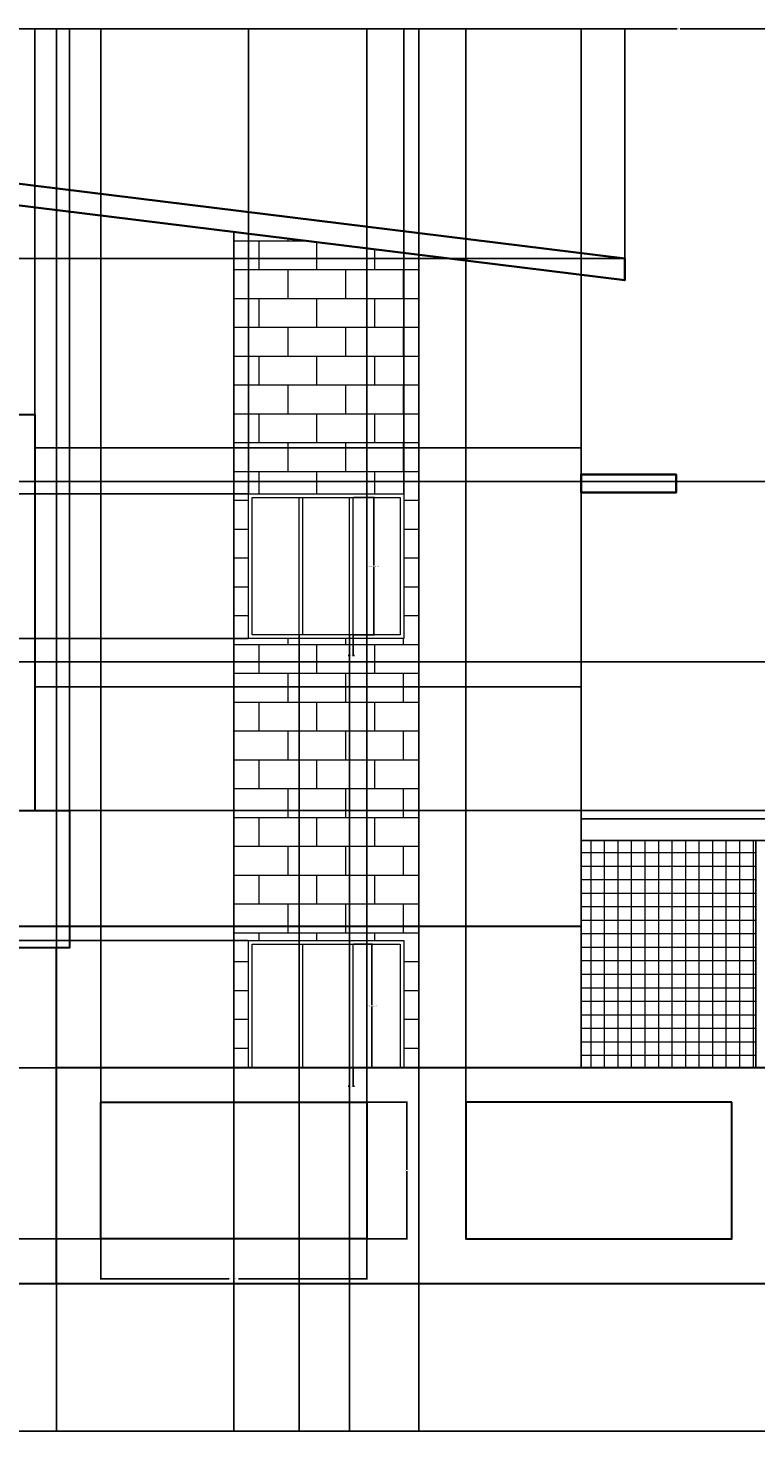
# Model space of a CAD drawing. Units: inches. Extents: x -14 to 886, y 45 to 435.
# Tile 4 of 5: x 384 to 586, y 45 to 435. Entities that reach past the tile are written whole.
import ezdxf

# ---------------------------------------------------------------- set-up
doc = ezdxf.new("R2010")
doc.units = ezdxf.units.IN
doc.header["$MEASUREMENT"] = 0
for name, color, linetype, lineweight in [('A-ANNO-DIMS', 2, 'Continuous', 18), ('A-ELEV-BAND', 7, 'Continuous', 30), ('A-ELEV-PATT', 252, 'Continuous', 13), ('A-GLAZ', 4, 'Continuous', 18), ('A-ROOF', 7, 'Continuous', 35), ('A-WALL', 7, 'Continuous', 25), ('A-WALL-PATT', 252, 'Continuous', 13), ('L-WALL', 7, 'Continuous', 30)]:
    doc.layers.add(name, color=color, linetype=linetype, lineweight=lineweight)
doc.styles.get("Standard").update_dxf_attribs({"font": 'arial.ttf'})
doc.dimstyles.get("Standard").update_dxf_attribs({"dimtxt": 0.18, "dimasz": 0.18, "dimexe": 0.18, "dimexo": 0.0625, "dimgap": 0.09, "dimtad": 0, "dimtih": 1, "dimtoh": 1, "dimdec": 4, "dimzin": 0, "dimdsep": 46, "dimtxsty": 'Standard', "dimcen": 0.09, "dimadec": 0, "dimazin": 0, "dimtfac": 1, "dimtdec": 4, "dimtofl": 0, "dimtmove": 0, "dimatfit": 3, "dimfxl": 1, "dimtolj": 1, "dimtzin": 0, "dimarcsym": 0})

# ---------------------------------------------------------------- blocks, each defined once
blk = doc.blocks.new('BOUNDARY-WALL-INSET')
blk.add_lwpolyline([(0, 37.91), (73.78, 37.91), (73.78, 0), (0, 0)], close=True)
blk = doc.blocks.new('MULLION-UPPER')
for p, q in [((0, 0), (0, 38.1)), ((1, 0), (1, 38.1))]:
    blk.add_line(p, q)
blk = doc.blocks.new('MULLION-LOWER')
for p, q in [((0, 0), (0, 34.29)), ((1, 0), (1, 34.29))]:
    blk.add_line(p, q)
blk = doc.blocks.new('*D10')
at = {"layer": 'A-ANNO-DIMS', "color": 0, "lineweight": -2, "transparency": 16777216}
for p, q in [((404.07, 99), (404.07, 87.81)), ((477.85, 99), (477.85, 87.81)), ((404.25, 87.99), (439.64, 87.99)), ((477.67, 87.99), (442.27, 87.99))]:
    blk.add_line(p, q, dxfattribs=at)
at = {"layer": 'A-ANNO-DIMS', "color": 0, "transparency": 16777216}
for points in [[(404.25, 88.02), (404.25, 87.96), (404.07, 87.99)], [(477.67, 88.02), (477.67, 87.96), (477.85, 87.99)]]:
    blk.add_solid(points, dxfattribs=at)
at = {"layer": 'Defpoints', "color": 0, "transparency": 16777216}
for p in [(404.07, 99.06), (477.85, 99.06), (477.85, 87.99)]:
    blk.add_point(p, dxfattribs=at)
at = {"layer": 'A-ANNO-DIMS', "color": 0, "transparency": 16777216, "insert": (440.96, 87.99), "char_height": 0.18, "attachment_point": 5}
blk.add_mtext('\\A1;WALL INSET 74 TYP.', dxfattribs=at)
blk = doc.blocks.new('*D11')
at = {"layer": 'A-ANNO-DIMS', "color": 0, "lineweight": -2, "transparency": 16777216}
for p, q in [((477.91, 136.97), (489.09, 136.97)), ((488.91, 136.79), (488.91, 118.2)), ((488.91, 99.24), (488.91, 117.83)), ((477.91, 99.06), (489.09, 99.06))]:
    blk.add_line(p, q, dxfattribs=at)
at = {"layer": 'A-ANNO-DIMS', "color": 0, "transparency": 16777216}
for points in [[(488.88, 136.79), (488.94, 136.79), (488.91, 136.97)], [(488.88, 99.24), (488.94, 99.24), (488.91, 99.06)]]:
    blk.add_solid(points, dxfattribs=at)
at = {"layer": 'Defpoints', "color": 0, "transparency": 16777216}
for p in [(477.85, 136.97), (488.91, 136.97), (477.85, 99.06)]:
    blk.add_point(p, dxfattribs=at)
at = {"layer": 'A-ANNO-DIMS', "color": 0, "transparency": 16777216, "insert": (488.91, 118.01), "char_height": 0.18, "attachment_point": 5}
blk.add_mtext('\\A1;38 TYP.', dxfattribs=at)
blk = doc.blocks.new('*D12')
at = {"layer": 'A-ANNO-DIMS', "color": 0, "lineweight": -2, "transparency": 16777216}
for p, q in [((474.11, 304.77), (479.94, 304.77)), ((479.76, 304.59), (479.76, 285.9)), ((479.76, 266.85), (479.76, 285.54)), ((474.11, 266.67), (479.94, 266.67))]:
    blk.add_line(p, q, dxfattribs=at)
at = {"layer": 'A-ANNO-DIMS', "color": 0, "transparency": 16777216}
for points in [[(479.73, 304.59), (479.79, 304.59), (479.76, 304.77)], [(479.73, 266.85), (479.79, 266.85), (479.76, 266.67)]]:
    blk.add_solid(points, dxfattribs=at)
at = {"layer": 'Defpoints', "color": 0, "transparency": 16777216}
for p in [(474.04, 304.77), (479.76, 304.77), (474.04, 266.67)]:
    blk.add_point(p, dxfattribs=at)
at = {"layer": 'A-ANNO-DIMS', "color": 0, "transparency": 16777216, "insert": (479.76, 285.72), "char_height": 0.18, "attachment_point": 5}
blk.add_mtext('\\A1;UPPER MULLION 38 TYP.', dxfattribs=at)
blk = doc.blocks.new('*D13')
at = {"layer": 'A-ANNO-DIMS', "color": 0, "lineweight": -2, "transparency": 16777216}
for p, q in [((473.04, 266.61), (473.04, 260.77)), ((474.04, 266.61), (474.04, 260.77)), ((472.86, 260.95), (472.68, 260.95)), ((474.22, 260.95), (474.4, 260.95))]:
    blk.add_line(p, q, dxfattribs=at)
at = {"layer": 'A-ANNO-DIMS', "color": 0, "transparency": 16777216}
for points in [[(472.86, 260.98), (472.86, 260.92), (473.04, 260.95)], [(474.22, 260.98), (474.22, 260.92), (474.04, 260.95)]]:
    blk.add_solid(points, dxfattribs=at)
at = {"layer": 'Defpoints', "color": 0, "transparency": 16777216}
for p in [(473.04, 266.67), (474.04, 266.67), (474.04, 260.95)]:
    blk.add_point(p, dxfattribs=at)
at = {"layer": 'A-ANNO-DIMS', "color": 0, "transparency": 16777216, "insert": (473.54, 260.95), "char_height": 0.18, "attachment_point": 5}
blk.add_mtext('\\A1;1 TYP.', dxfattribs=at)
blk = doc.blocks.new('*D14')
at = {"layer": 'A-ANNO-DIMS', "color": 0, "lineweight": -2, "transparency": 16777216}
for p, q in [((474.11, 180.83), (479.37, 180.83)), ((479.19, 180.65), (479.19, 163.87)), ((479.19, 146.72), (479.19, 163.5)), ((474.11, 146.54), (479.37, 146.54))]:
    blk.add_line(p, q, dxfattribs=at)
at = {"layer": 'A-ANNO-DIMS', "color": 0, "transparency": 16777216}
for points in [[(479.16, 180.65), (479.22, 180.65), (479.19, 180.83)], [(479.16, 146.72), (479.22, 146.72), (479.19, 146.54)]]:
    blk.add_solid(points, dxfattribs=at)
at = {"layer": 'Defpoints', "color": 0, "transparency": 16777216}
for p in [(474.04, 180.83), (479.19, 180.83), (474.04, 146.54)]:
    blk.add_point(p, dxfattribs=at)
at = {"layer": 'A-ANNO-DIMS', "color": 0, "transparency": 16777216, "insert": (479.19, 163.69), "char_height": 0.18, "attachment_point": 5}
blk.add_mtext('\\A1;LOWER MULLION 34 TYP.', dxfattribs=at)
blk = doc.blocks.new('*D15')
at = {"layer": 'A-ANNO-DIMS', "color": 0, "lineweight": -2, "transparency": 16777216}
for p, q in [((473.04, 146.48), (473.04, 141.21)), ((474.04, 146.48), (474.04, 141.21)), ((472.86, 141.39), (472.68, 141.39)), ((474.22, 141.39), (474.4, 141.39))]:
    blk.add_line(p, q, dxfattribs=at)
at = {"layer": 'A-ANNO-DIMS', "color": 0, "transparency": 16777216}
for points in [[(472.86, 141.42), (472.86, 141.36), (473.04, 141.39)], [(474.22, 141.42), (474.22, 141.36), (474.04, 141.39)]]:
    blk.add_solid(points, dxfattribs=at)
at = {"layer": 'Defpoints', "color": 0, "transparency": 16777216}
for p in [(473.04, 146.54), (474.04, 146.54), (474.04, 141.39)]:
    blk.add_point(p, dxfattribs=at)
at = {"layer": 'A-ANNO-DIMS', "color": 0, "transparency": 16777216, "insert": (473.54, 141.39), "char_height": 0.18, "attachment_point": 5}
blk.add_mtext('\\A1;1 TYP.', dxfattribs=at)
blk = doc.blocks.new('*D16')
at = {"layer": 'A-ANNO-DIMS', "color": 0, "lineweight": -2, "transparency": 16777216}
for p, q in [((111.3, 86.48), (111.3, 45.47)), ((591.3, 86.48), (591.3, 45.47)), ((111.48, 45.65), (351.01, 45.65)), ((591.12, 45.65), (351.59, 45.65))]:
    blk.add_line(p, q, dxfattribs=at)
at = {"layer": 'A-ANNO-DIMS', "color": 0, "transparency": 16777216}
for points in [[(111.48, 45.68), (111.48, 45.62), (111.3, 45.65)], [(591.12, 45.68), (591.12, 45.62), (591.3, 45.65)]]:
    blk.add_solid(points, dxfattribs=at)
at = {"layer": 'Defpoints', "color": 0, "transparency": 16777216}
for p in [(111.3, 86.54), (591.3, 86.54), (591.3, 45.65)]:
    blk.add_point(p, dxfattribs=at)
at = {"layer": 'A-ANNO-DIMS', "color": 0, "transparency": 16777216, "insert": (351.3, 45.65), "char_height": 0.18, "attachment_point": 5}
blk.add_mtext('\\A1;480', dxfattribs=at)
blk = doc.blocks.new('*D23')
at = {"layer": 'A-ANNO-DIMS', "color": 0, "lineweight": -2, "transparency": 16777216}
for p, q in [((379.79, 86.48), (379.79, 45.47)), ((391.79, 86.48), (391.79, 45.47)), ((379.97, 45.65), (385.58, 45.65)), ((391.61, 45.65), (386, 45.65))]:
    blk.add_line(p, q, dxfattribs=at)
at = {"layer": 'A-ANNO-DIMS', "color": 0, "transparency": 16777216}
for points in [[(379.97, 45.68), (379.97, 45.62), (379.79, 45.65)], [(391.61, 45.68), (391.61, 45.62), (391.79, 45.65)]]:
    blk.add_solid(points, dxfattribs=at)
at = {"layer": 'Defpoints', "color": 0, "transparency": 16777216}
for p in [(379.79, 86.54), (391.79, 86.54), (391.79, 45.65)]:
    blk.add_point(p, dxfattribs=at)
at = {"layer": 'A-ANNO-DIMS', "color": 0, "transparency": 16777216, "insert": (385.79, 45.65), "char_height": 0.18, "attachment_point": 5}
blk.add_mtext('\\A1;12', dxfattribs=at)
blk = doc.blocks.new('*D28')
at = {"layer": 'A-ANNO-DIMS', "color": 0, "lineweight": -2, "transparency": 16777216}
for p, q in [((364.23, 394.04), (364.23, 435.05)), ((364.41, 434.87), (456.34, 434.87)), ((549.17, 434.87), (457.25, 434.87)), ((549.35, 371.18), (549.35, 435.05))]:
    blk.add_line(p, q, dxfattribs=at)
at = {"layer": 'A-ANNO-DIMS', "color": 0, "transparency": 16777216}
for points in [[(364.41, 434.9), (364.41, 434.84), (364.23, 434.87)], [(549.17, 434.9), (549.17, 434.84), (549.35, 434.87)]]:
    blk.add_solid(points, dxfattribs=at)
at = {"layer": 'Defpoints', "color": 0, "transparency": 16777216}
for p in [(549.35, 434.87), (364.23, 393.98), (549.35, 371.11)]:
    blk.add_point(p, dxfattribs=at)
at = {"layer": 'A-ANNO-DIMS', "color": 0, "transparency": 16777216, "insert": (456.79, 434.87), "char_height": 0.18, "attachment_point": 5}
blk.add_mtext('\\A1;185.12', dxfattribs=at)
blk = doc.blocks.new('*D29')
at = {"layer": 'A-ANNO-DIMS', "color": 0, "lineweight": -2, "transparency": 16777216}
for p, q in [((364.17, 393.98), (-13.96, 393.98)), ((-13.78, 393.8), (-13.78, 382.73)), ((-13.78, 371.29), (-13.78, 382.37)), ((549.29, 371.11), (-13.96, 371.11))]:
    blk.add_line(p, q, dxfattribs=at)
at = {"layer": 'A-ANNO-DIMS', "color": 0, "transparency": 16777216}
for points in [[(-13.81, 393.8), (-13.75, 393.8), (-13.78, 393.98)], [(-13.81, 371.29), (-13.75, 371.29), (-13.78, 371.11)]]:
    blk.add_solid(points, dxfattribs=at)
at = {"layer": 'Defpoints', "color": 0, "transparency": 16777216}
for p in [(364.23, 393.98), (-13.78, 371.11), (549.35, 371.11)]:
    blk.add_point(p, dxfattribs=at)
at = {"layer": 'A-ANNO-DIMS', "color": 0, "transparency": 16777216, "insert": (-13.78, 382.55), "char_height": 0.18, "attachment_point": 5}
blk.add_mtext('\\A1;22.865', dxfattribs=at)
blk = doc.blocks.new('*D30')
at = {"layer": 'A-ANNO-DIMS', "color": 0, "lineweight": -2, "transparency": 16777216}
for p, q in [((537.25, 366.63), (537.25, 435.05)), ((537.43, 434.87), (542.85, 434.87)), ((549.17, 434.87), (543.76, 434.87)), ((549.35, 371.18), (549.35, 435.05))]:
    blk.add_line(p, q, dxfattribs=at)
at = {"layer": 'A-ANNO-DIMS', "color": 0, "transparency": 16777216}
for points in [[(537.43, 434.9), (537.43, 434.84), (537.25, 434.87)], [(549.17, 434.9), (549.17, 434.84), (549.35, 434.87)]]:
    blk.add_solid(points, dxfattribs=at)
at = {"layer": 'Defpoints', "color": 0, "transparency": 16777216}
for p in [(537.25, 434.87), (549.35, 371.11), (537.25, 366.56)]:
    blk.add_point(p, dxfattribs=at)
at = {"layer": 'A-ANNO-DIMS', "color": 0, "transparency": 16777216, "insert": (543.3, 434.87), "char_height": 0.18, "attachment_point": 5}
blk.add_mtext('\\A1;12.103', dxfattribs=at)
blk = doc.blocks.new('*D31')
at = {"layer": 'A-ANNO-DIMS', "color": 0, "lineweight": -2, "transparency": 16777216}
for p, q in [((303.24, 327.84), (303.24, 435.05)), ((303.42, 434.87), (344.12, 434.87)), ((385.61, 434.87), (344.91, 434.87)), ((385.79, 327.84), (385.79, 435.05))]:
    blk.add_line(p, q, dxfattribs=at)
at = {"layer": 'A-ANNO-DIMS', "color": 0, "transparency": 16777216}
for points in [[(303.42, 434.9), (303.42, 434.84), (303.24, 434.87)], [(385.61, 434.9), (385.61, 434.84), (385.79, 434.87)]]:
    blk.add_solid(points, dxfattribs=at)
at = {"layer": 'Defpoints', "color": 0, "transparency": 16777216}
for p in [(385.79, 434.87), (303.24, 327.78), (385.79, 327.78)]:
    blk.add_point(p, dxfattribs=at)
at = {"layer": 'A-ANNO-DIMS', "color": 0, "transparency": 16777216, "insert": (344.51, 434.87), "char_height": 0.18, "attachment_point": 5}
blk.add_mtext('\\A1;82.55', dxfattribs=at)
blk = doc.blocks.new('*D33')
at = {"layer": 'A-ANNO-DIMS', "color": 0, "lineweight": -2, "transparency": 16777216}
for p, q in [((385.79, 217.95), (385.79, 435.05)), ((385.97, 434.87), (390.17, 434.87)), ((395.16, 434.87), (390.96, 434.87)), ((395.34, 217.95), (395.34, 435.05))]:
    blk.add_line(p, q, dxfattribs=at)
at = {"layer": 'A-ANNO-DIMS', "color": 0, "transparency": 16777216}
for points in [[(385.97, 434.9), (385.97, 434.84), (385.79, 434.87)], [(395.16, 434.9), (395.16, 434.84), (395.34, 434.87)]]:
    blk.add_solid(points, dxfattribs=at)
at = {"layer": 'Defpoints', "color": 0, "transparency": 16777216}
for p in [(395.34, 434.87), (385.79, 217.88), (395.34, 217.88)]:
    blk.add_point(p, dxfattribs=at)
at = {"layer": 'A-ANNO-DIMS', "color": 0, "transparency": 16777216, "insert": (390.57, 434.87), "char_height": 0.18, "attachment_point": 5}
blk.add_mtext('\\A1;9.549', dxfattribs=at)
blk = doc.blocks.new('*D34')
at = {"layer": 'A-ANNO-DIMS', "color": 0, "lineweight": -2, "transparency": 16777216}
for p, q in [((177.3, 179.88), (177.3, 435.05)), ((177.48, 434.87), (285.86, 434.87)), ((395.16, 434.87), (286.79, 434.87)), ((395.34, 179.88), (395.34, 435.05))]:
    blk.add_line(p, q, dxfattribs=at)
at = {"layer": 'A-ANNO-DIMS', "color": 0, "transparency": 16777216}
for points in [[(177.48, 434.9), (177.48, 434.84), (177.3, 434.87)], [(395.16, 434.9), (395.16, 434.84), (395.34, 434.87)]]:
    blk.add_solid(points, dxfattribs=at)
at = {"layer": 'Defpoints', "color": 0, "transparency": 16777216}
for p in [(395.34, 434.87), (177.3, 179.82), (395.34, 179.82)]:
    blk.add_point(p, dxfattribs=at)
at = {"layer": 'A-ANNO-DIMS', "color": 0, "transparency": 16777216, "insert": (286.32, 434.87), "char_height": 0.18, "attachment_point": 5}
blk.add_mtext('\\A1;218.04', dxfattribs=at)
blk = doc.blocks.new('*D35')
at = {"layer": 'A-ANNO-DIMS', "color": 0, "lineweight": -2, "transparency": 16777216}
for p, q in [((395.28, 217.88), (-13.96, 217.88)), ((-13.78, 217.7), (-13.78, 199.03)), ((-13.78, 180), (-13.78, 198.67)), ((395.28, 179.82), (-13.96, 179.82))]:
    blk.add_line(p, q, dxfattribs=at)
at = {"layer": 'A-ANNO-DIMS', "color": 0, "transparency": 16777216}
for points in [[(-13.81, 217.7), (-13.75, 217.7), (-13.78, 217.88)], [(-13.81, 180), (-13.75, 180), (-13.78, 179.82)]]:
    blk.add_solid(points, dxfattribs=at)
at = {"layer": 'Defpoints', "color": 0, "transparency": 16777216}
for p in [(-13.78, 217.88), (395.34, 217.88), (395.34, 179.82)]:
    blk.add_point(p, dxfattribs=at)
at = {"layer": 'A-ANNO-DIMS', "color": 0, "transparency": 16777216, "insert": (-13.78, 198.85), "char_height": 0.18, "attachment_point": 5}
blk.add_mtext('\\A1;38.06', dxfattribs=at)
blk = doc.blocks.new('*D39')
at = {"layer": 'A-ANNO-DIMS', "color": 0, "lineweight": -2, "transparency": 16777216}
for p, q in [((492.22, 146.6), (492.22, 435.05)), ((492.4, 434.87), (514.34, 434.87)), ((537.07, 434.87), (515.13, 434.87)), ((537.25, 146.6), (537.25, 435.05))]:
    blk.add_line(p, q, dxfattribs=at)
at = {"layer": 'A-ANNO-DIMS', "color": 0, "transparency": 16777216}
for points in [[(492.4, 434.9), (492.4, 434.84), (492.22, 434.87)], [(537.07, 434.9), (537.07, 434.84), (537.25, 434.87)]]:
    blk.add_solid(points, dxfattribs=at)
at = {"layer": 'Defpoints', "color": 0, "transparency": 16777216}
for p in [(537.25, 434.87), (492.22, 146.54), (537.25, 146.54)]:
    blk.add_point(p, dxfattribs=at)
at = {"layer": 'A-ANNO-DIMS', "color": 0, "transparency": 16777216, "insert": (514.73, 434.87), "char_height": 0.18, "attachment_point": 5}
blk.add_mtext('\\A1;45.03', dxfattribs=at)
blk = doc.blocks.new('*D40')
at = {"layer": 'A-ANNO-DIMS', "color": 0, "lineweight": -2, "transparency": 16777216}
for p, q in [((537.25, 259.21), (537.25, 435.05)), ((537.43, 434.87), (563.88, 434.87)), ((591.12, 434.87), (564.67, 434.87)), ((591.3, 259.21), (591.3, 435.05))]:
    blk.add_line(p, q, dxfattribs=at)
at = {"layer": 'A-ANNO-DIMS', "color": 0, "transparency": 16777216}
for points in [[(537.43, 434.9), (537.43, 434.84), (537.25, 434.87)], [(591.12, 434.9), (591.12, 434.84), (591.3, 434.87)]]:
    blk.add_solid(points, dxfattribs=at)
at = {"layer": 'Defpoints', "color": 0, "transparency": 16777216}
for p in [(591.3, 434.87), (537.25, 259.14), (591.3, 259.14)]:
    blk.add_point(p, dxfattribs=at)
at = {"layer": 'A-ANNO-DIMS', "color": 0, "transparency": 16777216, "insert": (564.28, 434.87), "char_height": 0.18, "attachment_point": 5}
blk.add_mtext('\\A1;54.05', dxfattribs=at)
blk = doc.blocks.new('*D41')
at = {"layer": 'A-ANNO-DIMS', "color": 0, "lineweight": -2, "transparency": 16777216}
for p, q in [((591.24, 259.14), (-13.96, 259.14)), ((-13.78, 258.96), (-13.78, 203.02)), ((-13.78, 146.72), (-13.78, 202.66)), ((537.19, 146.54), (-13.96, 146.54))]:
    blk.add_line(p, q, dxfattribs=at)
at = {"layer": 'A-ANNO-DIMS', "color": 0, "transparency": 16777216}
for points in [[(-13.81, 258.96), (-13.75, 258.96), (-13.78, 259.14)], [(-13.81, 146.72), (-13.75, 146.72), (-13.78, 146.54)]]:
    blk.add_solid(points, dxfattribs=at)
at = {"layer": 'Defpoints', "color": 0, "transparency": 16777216}
for p in [(-13.78, 259.14), (591.3, 259.14), (537.25, 146.54)]:
    blk.add_point(p, dxfattribs=at)
at = {"layer": 'A-ANNO-DIMS', "color": 0, "transparency": 16777216, "insert": (-13.78, 202.84), "char_height": 0.18, "attachment_point": 5}
blk.add_mtext('\\A1;112.6', dxfattribs=at)
blk = doc.blocks.new('*D51')
at = {"layer": 'A-ANNO-DIMS', "color": 0, "lineweight": -2, "transparency": 16777216}
for p, q in [((370.91, 309.22), (885.58, 309.22)), ((885.4, 309.04), (885.4, 263.74)), ((885.4, 218.06), (885.4, 263.37)), ((370.91, 217.88), (885.58, 217.88))]:
    blk.add_line(p, q, dxfattribs=at)
at = {"layer": 'A-ANNO-DIMS', "color": 0, "transparency": 16777216}
for points in [[(885.37, 309.04), (885.43, 309.04), (885.4, 309.22)], [(885.37, 218.06), (885.43, 218.06), (885.4, 217.88)]]:
    blk.add_solid(points, dxfattribs=at)
at = {"layer": 'Defpoints', "color": 0, "transparency": 16777216}
for p in [(370.85, 309.22), (885.4, 309.22), (370.85, 217.88)]:
    blk.add_point(p, dxfattribs=at)
at = {"layer": 'A-ANNO-DIMS', "color": 0, "transparency": 16777216, "insert": (885.4, 263.55), "char_height": 0.18, "attachment_point": 5}
blk.add_mtext('\\A1;91.34', dxfattribs=at)
blk = doc.blocks.new('*D52')
at = {"layer": 'A-ANNO-DIMS', "color": 0, "lineweight": -2, "transparency": 16777216}
for p, q in [((445.04, 305.84), (445.04, 435.05)), ((445.22, 434.87), (466.16, 434.87)), ((487.87, 434.87), (466.92, 434.87)), ((488.05, 305.84), (488.05, 435.05))]:
    blk.add_line(p, q, dxfattribs=at)
at = {"layer": 'A-ANNO-DIMS', "color": 0, "transparency": 16777216}
for points in [[(445.22, 434.9), (445.22, 434.84), (445.04, 434.87)], [(487.87, 434.9), (487.87, 434.84), (488.05, 434.87)]]:
    blk.add_solid(points, dxfattribs=at)
at = {"layer": 'Defpoints', "color": 0, "transparency": 16777216}
for p in [(488.05, 434.87), (445.04, 305.77), (488.05, 305.77)]:
    blk.add_point(p, dxfattribs=at)
at = {"layer": 'A-ANNO-DIMS', "color": 0, "transparency": 16777216, "insert": (466.54, 434.87), "char_height": 0.18, "attachment_point": 5}
blk.add_mtext('\\A1;43.01', dxfattribs=at)
blk = doc.blocks.new('*D53')
at = {"layer": 'A-ANNO-DIMS', "color": 0, "lineweight": -2, "transparency": 16777216}
for p, q in [((444.97, 305.77), (-13.96, 305.77)), ((-13.78, 305.59), (-13.78, 285.9)), ((-13.78, 265.85), (-13.78, 285.54)), ((444.97, 265.67), (-13.96, 265.67))]:
    blk.add_line(p, q, dxfattribs=at)
at = {"layer": 'A-ANNO-DIMS', "color": 0, "transparency": 16777216}
for points in [[(-13.81, 305.59), (-13.75, 305.59), (-13.78, 305.77)], [(-13.81, 265.85), (-13.75, 265.85), (-13.78, 265.67)]]:
    blk.add_solid(points, dxfattribs=at)
at = {"layer": 'Defpoints', "color": 0, "transparency": 16777216}
for p in [(-13.78, 305.77), (445.04, 305.77), (445.04, 265.67)]:
    blk.add_point(p, dxfattribs=at)
at = {"layer": 'A-ANNO-DIMS', "color": 0, "transparency": 16777216, "insert": (-13.78, 285.72), "char_height": 0.18, "attachment_point": 5}
blk.add_mtext('\\A1;40.104', dxfattribs=at)
blk = doc.blocks.new('*D54')
at = {"layer": 'A-ANNO-DIMS', "color": 0, "lineweight": -2, "transparency": 16777216}
for p, q in [((444.97, 181.83), (-13.96, 181.83)), ((-13.78, 181.65), (-13.78, 164.37)), ((-13.78, 146.72), (-13.78, 164)), ((444.97, 146.54), (-13.96, 146.54))]:
    blk.add_line(p, q, dxfattribs=at)
at = {"layer": 'A-ANNO-DIMS', "color": 0, "transparency": 16777216}
for points in [[(-13.81, 181.65), (-13.75, 181.65), (-13.78, 181.83)], [(-13.81, 146.72), (-13.75, 146.72), (-13.78, 146.54)]]:
    blk.add_solid(points, dxfattribs=at)
at = {"layer": 'Defpoints', "color": 0, "transparency": 16777216}
for p in [(-13.78, 181.83), (445.04, 181.83), (445.04, 146.54)]:
    blk.add_point(p, dxfattribs=at)
at = {"layer": 'A-ANNO-DIMS', "color": 0, "transparency": 16777216, "insert": (-13.78, 164.19), "char_height": 0.18, "attachment_point": 5}
blk.add_mtext('\\A1;35.29', dxfattribs=at)
blk = doc.blocks.new('*D55')
at = {"layer": 'A-ANNO-DIMS', "color": 0, "lineweight": -2, "transparency": 16777216}
for p, q in [((444.97, 265.67), (-13.96, 265.67)), ((-13.78, 265.49), (-13.78, 223.93)), ((-13.78, 182.01), (-13.78, 223.57)), ((444.97, 181.83), (-13.96, 181.83))]:
    blk.add_line(p, q, dxfattribs=at)
at = {"layer": 'A-ANNO-DIMS', "color": 0, "transparency": 16777216}
for points in [[(-13.81, 265.49), (-13.75, 265.49), (-13.78, 265.67)], [(-13.81, 182.01), (-13.75, 182.01), (-13.78, 181.83)]]:
    blk.add_solid(points, dxfattribs=at)
at = {"layer": 'Defpoints', "color": 0, "transparency": 16777216}
for p in [(-13.78, 265.67), (445.04, 265.67), (445.04, 181.83)]:
    blk.add_point(p, dxfattribs=at)
at = {"layer": 'A-ANNO-DIMS', "color": 0, "transparency": 16777216, "insert": (-13.78, 223.75), "char_height": 0.18, "attachment_point": 5}
blk.add_mtext('\\A1;83.84', dxfattribs=at)
blk = doc.blocks.new('*D56')
at = {"layer": 'A-ANNO-DIMS', "color": 0, "lineweight": -2, "transparency": 16777216}
for p, q in [((440.96, 146.48), (440.96, 45.47)), ((492.22, 146.48), (492.22, 45.47)), ((441.14, 45.65), (466.19, 45.65)), ((492.04, 45.65), (466.98, 45.65))]:
    blk.add_line(p, q, dxfattribs=at)
at = {"layer": 'A-ANNO-DIMS', "color": 0, "transparency": 16777216}
for points in [[(441.14, 45.68), (441.14, 45.62), (440.96, 45.65)], [(492.04, 45.68), (492.04, 45.62), (492.22, 45.65)]]:
    blk.add_solid(points, dxfattribs=at)
at = {"layer": 'Defpoints', "color": 0, "transparency": 16777216}
for p in [(440.96, 146.54), (492.22, 146.54), (492.22, 45.65)]:
    blk.add_point(p, dxfattribs=at)
at = {"layer": 'A-ANNO-DIMS', "color": 0, "transparency": 16777216, "insert": (466.59, 45.65), "char_height": 0.18, "attachment_point": 5}
blk.add_mtext('\\A1;51.26', dxfattribs=at)
blk = doc.blocks.new('*D57')
at = {"layer": 'A-ANNO-DIMS', "color": 0, "lineweight": -2, "transparency": 16777216}
for p, q in [((404, 99.06), (-13.96, 99.06)), ((-13.78, 98.88), (-13.78, 92.98)), ((-13.78, 86.72), (-13.78, 92.62)), ((391.73, 86.54), (-13.96, 86.54))]:
    blk.add_line(p, q, dxfattribs=at)
at = {"layer": 'A-ANNO-DIMS', "color": 0, "transparency": 16777216}
for points in [[(-13.81, 98.88), (-13.75, 98.88), (-13.78, 99.06)], [(-13.81, 86.72), (-13.75, 86.72), (-13.78, 86.54)]]:
    blk.add_solid(points, dxfattribs=at)
at = {"layer": 'Defpoints', "color": 0, "transparency": 16777216}
for p in [(404.07, 99.06), (-13.78, 86.54), (391.79, 86.54)]:
    blk.add_point(p, dxfattribs=at)
at = {"layer": 'A-ANNO-DIMS', "color": 0, "transparency": 16777216, "insert": (-13.78, 92.8), "char_height": 0.18, "attachment_point": 5}
blk.add_mtext('\\A1;12.52', dxfattribs=at)
blk = doc.blocks.new('*D58')
at = {"layer": 'A-ANNO-DIMS', "color": 0, "lineweight": -2, "transparency": 16777216}
for p, q in [((391.79, 146.6), (391.79, 435.05)), ((391.97, 434.87), (397.47, 434.87)), ((403.89, 434.87), (398.38, 434.87)), ((404.07, 137.03), (404.07, 435.05))]:
    blk.add_line(p, q, dxfattribs=at)
at = {"layer": 'A-ANNO-DIMS', "color": 0, "transparency": 16777216}
for points in [[(391.97, 434.9), (391.97, 434.84), (391.79, 434.87)], [(403.89, 434.9), (403.89, 434.84), (404.07, 434.87)]]:
    blk.add_solid(points, dxfattribs=at)
at = {"layer": 'Defpoints', "color": 0, "transparency": 16777216}
for p in [(404.07, 434.87), (391.79, 146.54), (404.07, 136.97)]:
    blk.add_point(p, dxfattribs=at)
at = {"layer": 'A-ANNO-DIMS', "color": 0, "transparency": 16777216, "insert": (397.93, 434.87), "char_height": 0.18, "attachment_point": 5}
blk.add_mtext('\\A1;12.275', dxfattribs=at)
blk = doc.blocks.new('*D59')
at = {"layer": 'A-ANNO-DIMS', "color": 0, "lineweight": -2, "transparency": 16777216}
for p, q in [((477.85, 99.12), (477.85, 435.05)), ((478.03, 434.87), (491.22, 434.87)), ((505.07, 434.87), (491.87, 434.87)), ((505.25, 99.12), (505.25, 435.05))]:
    blk.add_line(p, q, dxfattribs=at)
at = {"layer": 'A-ANNO-DIMS', "color": 0, "transparency": 16777216}
for points in [[(478.03, 434.9), (478.03, 434.84), (477.85, 434.87)], [(505.07, 434.9), (505.07, 434.84), (505.25, 434.87)]]:
    blk.add_solid(points, dxfattribs=at)
at = {"layer": 'Defpoints', "color": 0, "transparency": 16777216}
for p in [(505.25, 434.87), (477.85, 99.06), (505.25, 99.06)]:
    blk.add_point(p, dxfattribs=at)
at = {"layer": 'A-ANNO-DIMS', "color": 0, "transparency": 16777216, "insert": (491.55, 434.87), "char_height": 0.18, "attachment_point": 5}
blk.add_mtext('\\A1;27.4', dxfattribs=at)
blk = doc.blocks.new('*D67')
at = {"layer": 'A-ANNO-DIMS', "color": 0, "lineweight": -2, "transparency": 16777216}
for p, q in [((459.04, 266.61), (459.04, 45.47)), ((473.04, 266.61), (473.04, 45.47)), ((459.22, 45.65), (465.59, 45.65)), ((472.86, 45.65), (466.5, 45.65))]:
    blk.add_line(p, q, dxfattribs=at)
at = {"layer": 'A-ANNO-DIMS', "color": 0, "transparency": 16777216}
for points in [[(459.22, 45.68), (459.22, 45.62), (459.04, 45.65)], [(472.86, 45.68), (472.86, 45.62), (473.04, 45.65)]]:
    blk.add_solid(points, dxfattribs=at)
at = {"layer": 'Defpoints', "color": 0, "transparency": 16777216}
for p in [(459.04, 266.67), (473.04, 266.67), (473.04, 45.65)]:
    blk.add_point(p, dxfattribs=at)
at = {"layer": 'A-ANNO-DIMS', "color": 0, "transparency": 16777216, "insert": (466.04, 45.65), "char_height": 0.18, "attachment_point": 5}
blk.add_mtext('\\A1;14.003', dxfattribs=at)

msp = doc.modelspace()

# ---------------------------------------------------------------- hatches: boundary and pattern name
at = {"layer": 'A-ELEV-PATT'}
h = msp.add_hatch(dxfattribs=at)
h.set_pattern_fill('NET', color=256, scale=30, style=0)
h.paths.add_polyline_path([(585.6689, 209.6038), (585.6689, 146.5389), (537.2506, 146.5389), (537.2506, 209.6038)])
at = {"layer": 'A-WALL-PATT'}
h = msp.add_hatch(dxfattribs=at)
h.set_pattern_fill('AR-B816', color=256, style=0)
h.paths.add_polyline_path([(440.9564, 378.4573), (440.9564, 146.5389), (445.0372, 146.5389), (445.0372, 181.8319), (488.0457, 181.8319), (488.0457, 146.5389), (492.2168, 146.5389), (492.2168, 372.1259)])
h.paths.add_polyline_path([(488.0457, 305.7727), (488.0457, 265.6686), (445.0372, 265.6686), (445.0372, 305.7727)], flags=0)

# ---------------------------------------------------------------- linework, layer by layer
at = {"layer": 'A-ELEV-BAND'}
for points in [[(303.2386, 327.7815), (303.2386, 217.8839), (303.2386, 327.7815), (385.7908, 327.7815), (385.7908, 217.8839)], [(379.7908, 217.8839), (379.7908, 319.7815), (309.2386, 319.7815), (309.2386, 217.8839), (395.3394, 217.8839), (395.3394, 179.8201), (177.3024, 179.8201)], [(177.3024, 185.8201), (395.3394, 185.8201), (537.2506, 185.8201)]]:
    msp.add_lwpolyline(points, dxfattribs=at)
at = {"layer": 'A-GLAZ'}
for points in [[(488.0457, 305.7727), (488.0457, 265.6686), (445.0372, 265.6686), (445.0372, 305.7727)], [(487.0457, 304.7727), (487.0457, 266.6686), (446.0372, 266.6686), (446.0372, 304.7727)]]:
    msp.add_lwpolyline(points, close=True, dxfattribs=at)
for points in [[(445.0372, 146.5389), (445.0372, 181.8319), (488.0457, 181.8319), (488.0457, 146.5389)], [(446.0372, 146.5389), (446.0372, 180.8319), (487.0457, 180.8319), (487.0457, 146.5389)]]:
    msp.add_lwpolyline(points, dxfattribs=at)
at = {"layer": 'A-ROOF'}
for points in [[(364.2304, 387.9341), (364.2304, 393.9797), (549.3534, 371.1143), (549.3534, 365.0687)], [(537.2506, 306.1411), (563.5875, 306.1411), (563.5875, 311.1871), (537.2506, 311.1871)]]:
    msp.add_lwpolyline(points, close=True, dxfattribs=at)
at = {"layer": 'A-WALL'}
for p, q in [((385.7908, 318.6087), (537.2506, 318.6087)), ((385.7908, 252.2144), (537.2506, 252.2144)), ((537.2506, 215.6038), (591.3024, 215.6038))]:
    msp.add_line(p, q, dxfattribs=at)
for points in [[(440.9564, 378.4573), (440.9564, 146.5389), (492.2168, 146.5389), (492.2168, 372.1259)], [(492.2168, 146.5389), (537.2506, 146.5389), (537.2506, 366.5636)], [(585.6689, 209.6038), (585.6689, 146.5389), (537.2506, 146.5389), (537.2506, 209.6038), (591.3024, 209.6038)]]:
    msp.add_lwpolyline(points, dxfattribs=at)
msp.add_lwpolyline([(591.3024, 215.6038), (537.2506, 215.6038), (537.2506, 259.1435), (591.3024, 259.1435)], close=True, dxfattribs=at)
at = {"layer": 'A-WALL-PATT'}
for points in [[(456, 312), (456, 318.6087), (456, 320)], [(472, 312), (472, 318.6087), (472, 320)], [(488, 312), (488, 318.6087), (488, 320)], [(456, 248), (456, 252.2144), (456, 256)], [(472, 248), (472, 252.2144), (472, 256)], [(488, 248), (488, 252.2144), (488, 256)], [(456, 184), (456, 185.8201), (456, 192)], [(472, 184), (472, 185.8201), (472, 192)], [(488, 184), (488, 185.8201), (488, 192)]]:
    msp.add_lwpolyline(points, dxfattribs=at)
at = {"layer": 'L-WALL'}
for p, q in [((391.7908, 86.5389), (391.7908, 179.8201)), ((591.3024, 146.5389), (391.7908, 146.5389)), ((591.3024, 86.5389), (379.7908, 86.5389))]:
    msp.add_line(p, q, dxfattribs=at)

# ---------------------------------------------------------------- block references
at = {"layer": 'A-GLAZ'}
for name, p in [('MULLION-UPPER', (459.04, 266.6686)), ('MULLION-UPPER', (473.0428, 266.6686)), ('MULLION-LOWER', (459.04, 146.5389)), ('MULLION-LOWER', (473.0428, 146.5389))]:
    msp.add_blockref(name, p, dxfattribs=at)
at = {"layer": 'L-WALL'}
msp.add_blockref('BOUNDARY-WALL-INSET', (404.0655, 99.0583), dxfattribs=at)
at = {"layer": 'L-WALL', "extrusion": (0, 0, -1), "zscale": -1}
msp.add_blockref('BOUNDARY-WALL-INSET', (-579.0277, 99.0583), dxfattribs=at)

# ---------------------------------------------------------------- dimensions: what is measured, and where the dimension line sits
at = {"layer": 'A-ANNO-DIMS'}
for base, p1, p2, override, picture, middle in [((395.3394, 434.8697), (177.3024, 179.8201), (395.3394, 179.8201), {"dimdec": 2, "dimlfac": 1, "dimrnd": 0, "dimzin": 0, "dimdsep": 46, "dimlunit": 2}, '*D34', (286.3209, 434.8697)), ((385.7908, 434.8697), (303.2386, 327.7815), (385.7908, 327.7815), {"dimdec": 2, "dimlfac": 1, "dimrnd": 0, "dimzin": 0, "dimdsep": 46, "dimlunit": 2}, '*D31', (344.5147, 434.8697)), ((549.3534, 434.8697), (364.2304, 393.9797), (549.3534, 371.1143), {"dimdec": 2, "dimlfac": 1, "dimrnd": 0, "dimzin": 0, "dimdsep": 46, "dimlunit": 2}, '*D28', (456.7919, 434.8697)), ((395.3394, 434.8697), (385.7908, 217.8839), (395.3394, 217.8839), {"dimdec": 3, "dimlfac": 1, "dimrnd": 0, "dimzin": 0, "dimdsep": 46, "dimlunit": 2}, '*D33', (390.5651, 434.8697)), ((404.0655, 434.8697), (391.7908, 146.5389), (404.0655, 136.9681), {"dimdec": 3, "dimlfac": 1, "dimrnd": 0, "dimzin": 0, "dimdsep": 46, "dimlunit": 2}, '*D58', (397.9282, 434.8697)), ((488.0457, 434.8697), (445.0372, 305.7727), (488.0457, 305.7727), {"dimdec": 2, "dimlfac": 1, "dimrnd": 0, "dimzin": 0, "dimdsep": 46, "dimlunit": 2}, '*D52', (466.5414, 434.8697)), ((505.2459, 434.8697), (477.8473, 99.0583), (505.2459, 99.0583), {"dimdec": 1, "dimlfac": 1, "dimrnd": 0, "dimzin": 0, "dimdsep": 46, "dimlunit": 2}, '*D59', (491.5466, 434.8697)), ((537.2506, 434.8697), (492.2168, 146.5389), (537.2506, 146.5389), {"dimdec": 2, "dimlfac": 1, "dimrnd": 0, "dimzin": 0, "dimdsep": 46, "dimlunit": 2}, '*D39', (514.7337, 434.8697)), ((537.2506, 434.8697), (549.3534, 371.1143), (537.2506, 366.5636), {"dimdec": 3, "dimlfac": 1, "dimrnd": 0, "dimzin": 0, "dimdsep": 46, "dimlunit": 2}, '*D30', (543.302, 434.8697)), ((591.3024, 434.8697), (537.2506, 259.1435), (591.3024, 259.1435), {"dimdec": 2, "dimlfac": 1, "dimrnd": 0, "dimzin": 0, "dimdsep": 46, "dimlunit": 2}, '*D40', (564.2765, 434.8697)), ((473.0428, 45.6489), (459.04, 266.6686), (473.0428, 266.6686), {"dimdec": 3, "dimlfac": 1, "dimrnd": 0, "dimzin": 0, "dimdsep": 46, "dimlunit": 2}, '*D67', (466.0414, 45.6489)), ((492.2168, 45.6489), (440.9564, 146.5389), (492.2168, 146.5389), {"dimdec": 2, "dimlfac": 1, "dimrnd": 0, "dimzin": 0, "dimdsep": 46, "dimlunit": 2}, '*D56', (466.5866, 45.6489)), ((591.3024, 45.6489), (111.3024, 86.5389), (591.3024, 86.5389), {"dimdec": 0, "dimlfac": 1, "dimrnd": 0, "dimzin": 0, "dimdsep": 46, "dimlunit": 2}, '*D16', (351.3024, 45.6489)), ((391.7908, 45.6489), (379.7908, 86.5389), (391.7908, 86.5389), {"dimdec": 0, "dimlfac": 1, "dimrnd": 0, "dimzin": 0, "dimdsep": 46, "dimlunit": 2}, '*D23', (385.7908, 45.6489))]:
    dim = msp.add_linear_dim(base=base, p1=p1, p2=p2, dimstyle='Standard', override=override, dxfattribs=at)
    dim.commit()
    dim.dimension.update_dxf_attribs({"geometry": picture, "text_midpoint": middle})
for base, p1, p2, override, picture, middle in [((-13.7769, 371.1143), (364.2304, 393.9797), (549.3534, 371.1143), {"dimdec": 3, "dimlfac": 1, "dimrnd": 0, "dimzin": 0, "dimdsep": 46, "dimlunit": 2}, '*D29', (-13.7769, 382.547)), ((885.401, 309.2241), (370.8507, 217.8839), (370.8507, 309.2241), {"dimdec": 2, "dimlfac": 1, "dimrnd": 0, "dimzin": 0, "dimdsep": 46, "dimlunit": 2}, '*D51', (885.401, 263.554)), ((-13.7769, 305.7727), (445.0372, 265.6686), (445.0372, 305.7727), {"dimdec": 3, "dimlfac": 1, "dimrnd": 0, "dimzin": 0, "dimdsep": 46, "dimlunit": 2}, '*D53', (-13.7769, 285.7207)), ((-13.7769, 265.6686), (445.0372, 181.8319), (445.0372, 265.6686), {"dimdec": 2, "dimlfac": 1, "dimrnd": 0, "dimzin": 0, "dimdsep": 46, "dimlunit": 2}, '*D55', (-13.7769, 223.7503)), ((-13.7769, 259.1435), (537.2506, 146.5389), (591.3024, 259.1435), {"dimdec": 1, "dimlfac": 1, "dimrnd": 0, "dimzin": 0, "dimdsep": 46, "dimlunit": 2}, '*D41', (-13.7769, 202.8412)), ((-13.7769, 217.8839), (395.3394, 179.8201), (395.3394, 217.8839), {"dimdec": 2, "dimlfac": 1, "dimrnd": 0, "dimzin": 0, "dimdsep": 46, "dimlunit": 2}, '*D35', (-13.7769, 198.852)), ((-13.7769, 181.8319), (445.0372, 146.5389), (445.0372, 181.8319), {"dimdec": 2, "dimlfac": 1, "dimrnd": 0, "dimzin": 0, "dimdsep": 46, "dimlunit": 2}, '*D54', (-13.7769, 164.1854)), ((-13.7769, 86.5389), (404.0655, 99.0583), (391.7908, 86.5389), {"dimdec": 2, "dimlfac": 1, "dimrnd": 0, "dimzin": 0, "dimdsep": 46, "dimlunit": 2}, '*D57', (-13.7769, 92.7986))]:
    dim = msp.add_linear_dim(base=base, p1=p1, p2=p2, angle=90, dimstyle='Standard', override=override, dxfattribs=at)
    dim.commit()
    dim.dimension.update_dxf_attribs({"geometry": picture, "text_midpoint": middle})
for base, p1, p2, text, picture, middle in [((479.7584, 304.7727), (474.0428, 266.6686), (474.0428, 304.7727), 'UPPER MULLION <> TYP.', '*D12', (479.7584, 285.7207)), ((479.1868, 180.8319), (474.0428, 146.5389), (474.0428, 180.8319), 'LOWER MULLION <> TYP.', '*D14', (479.1868, 163.6854)), ((488.9146, 136.9681), (477.8473, 99.0583), (477.8473, 136.9681), '<> TYP.', '*D11', (488.9146, 118.0132))]:
    dim = msp.add_linear_dim(base=base, p1=p1, p2=p2, angle=90, text=text, dimstyle='Standard', override={"dimdec": 0, "dimlfac": 1, "dimrnd": 0, "dimzin": 0, "dimdsep": 46, "dimlunit": 2}, dxfattribs=at)
    dim.commit()
    dim.dimension.update_dxf_attribs({"geometry": picture, "text_midpoint": middle})
for base, p1, p2, text, picture, middle in [((474.0428, 260.953), (473.0428, 266.6686), (474.0428, 266.6686), '<> TYP.', '*D13', (473.5428, 260.953)), ((474.0428, 141.3949), (473.0428, 146.5389), (474.0428, 146.5389), '<> TYP.', '*D15', (473.5428, 141.3949)), ((477.8473, 87.991), (404.0655, 99.0583), (477.8473, 99.0583), 'WALL INSET <> TYP.', '*D10', (440.9564, 87.991))]:
    dim = msp.add_linear_dim(base=base, p1=p1, p2=p2, text=text, dimstyle='Standard', override={"dimdec": 0, "dimlfac": 1, "dimrnd": 0, "dimzin": 0, "dimdsep": 46, "dimlunit": 2}, dxfattribs=at)
    dim.commit()
    dim.dimension.update_dxf_attribs({"geometry": picture, "text_midpoint": middle})

doc.saveas('drawing.dxf')
